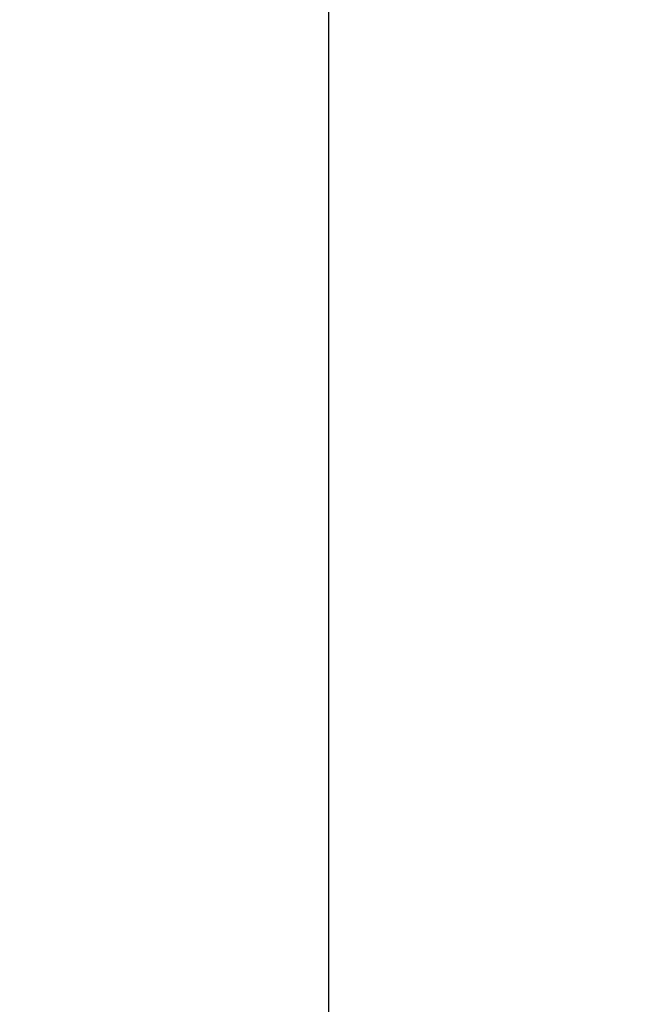
# Model space of a CAD drawing. Units: inches. Extents: x -5 to 482, y -460 to 66.
# Tile 25 of 31: x 72.83 to 84.19, y -28.5 to -10.4. Entities that reach past the tile are written whole.
import ezdxf

# ---------------------------------------------------------------- set-up
doc = ezdxf.new("R2010")
doc.units = ezdxf.units.IN
doc.header["$MEASUREMENT"] = 0
doc.layers.add('A-ANNO-DIMS', color=2, linetype='Continuous', lineweight=18)
doc.styles.get("Standard").update_dxf_attribs({"font": 'arial.ttf'})
doc.dimstyles.get("Standard").update_dxf_attribs({"dimtxt": 0.18, "dimasz": 0.18, "dimexe": 0.18, "dimexo": 0.0625, "dimgap": 0.09, "dimtad": 0, "dimtih": 1, "dimtoh": 1, "dimdec": 0, "dimzin": 0, "dimdsep": 46, "dimlunit": 3, "dimtxsty": 'Standard', "dimcen": 0.09, "dimadec": 0, "dimazin": 0, "dimtfac": 1, "dimtdec": 0, "dimtofl": 0, "dimtmove": 0, "dimatfit": 3, "dimfxl": 1, "dimtolj": 1, "dimtzin": 0, "dimarcsym": 0})

# ---------------------------------------------------------------- blocks, each defined once
blk = doc.blocks.new('*D6')
at = {"layer": 'A-ANNO-DIMS', "color": 0, "lineweight": -2, "transparency": 16777216}
for p, q in [((78.657, 4.151), (78.326, 4.151)), ((78.506, 3.971), (78.506, -64.746)), ((78.506, -139.669), (78.506, -70.951)), ((78.657, -139.849), (78.326, -139.849))]:
    blk.add_line(p, q, dxfattribs=at)
at = {"layer": 'A-ANNO-DIMS', "color": 0, "transparency": 16777216}
for points in [[(78.476, 3.971), (78.536, 3.971), (78.506, 4.151)], [(78.476, -139.669), (78.536, -139.669), (78.506, -139.849)]]:
    blk.add_solid(points, dxfattribs=at)
at = {"layer": 'Defpoints', "color": 0, "transparency": 16777216}
for p in [(78.72, 4.151), (78.506, -139.849), (78.72, -139.849)]:
    blk.add_point(p, dxfattribs=at)
at = {"layer": 'A-ANNO-DIMS', "color": 0, "transparency": 16777216, "insert": (78.506, -67.849), "char_height": 6, "attachment_point": 5}
blk.add_mtext("\\A1;12'", dxfattribs=at)

msp = doc.modelspace()

# ---------------------------------------------------------------- dimensions: what is measured, and where the dimension line sits
at = {"layer": 'A-ANNO-DIMS'}
dim = msp.add_linear_dim(base=(78.506, -139.849), p1=(78.72, 4.151), p2=(78.72, -139.849), angle=90, dimstyle='Standard', override={"dimtxt": 6, "dimclrd": 0, "dimclre": 0, "dimclrt": 0}, dxfattribs=at)
dim.commit()
dim.dimension.update_dxf_attribs({"geometry": '*D6', "text_midpoint": (78.506, -67.849)})

doc.saveas('drawing.dxf')
